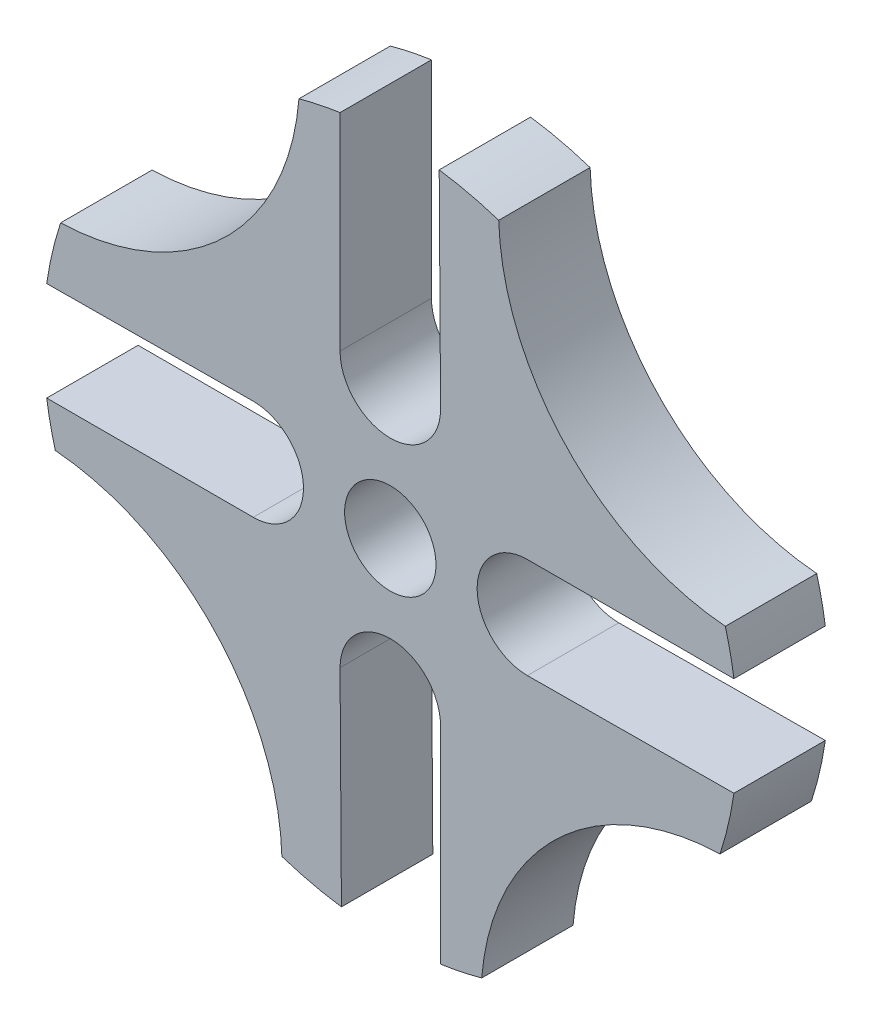
ISO-10303-21;
HEADER;
FILE_DESCRIPTION(('STEP AP214'),'2;1');
FILE_NAME('part.step','',(''),(''),'','','');
FILE_SCHEMA(('AUTOMOTIVE_DESIGN { 1 0 10303 214 1 1 1 1 }'));
ENDSEC;
DATA;
#1=APPLICATION_CONTEXT('core data for automotive mechanical design processes');
#2=APPLICATION_PROTOCOL_DEFINITION('international standard','automotive_design',2000,#1);
#3=PRODUCT_CONTEXT('',#1,'mechanical');
#4=PRODUCT('Part','Part','',(#3));
#5=PRODUCT_RELATED_PRODUCT_CATEGORY('part','',(#4));
#6=PRODUCT_DEFINITION_FORMATION('','',#4);
#7=PRODUCT_DEFINITION_CONTEXT('part definition',#1,'design');
#8=PRODUCT_DEFINITION('design','',#6,#7);
#9=PRODUCT_DEFINITION_SHAPE('','',#8);
#10=(LENGTH_UNIT() NAMED_UNIT(*) SI_UNIT(.MILLI.,.METRE.));
#11=(NAMED_UNIT(*) PLANE_ANGLE_UNIT() SI_UNIT($,.RADIAN.));
#12=(NAMED_UNIT(*) SI_UNIT($,.STERADIAN.) SOLID_ANGLE_UNIT());
#13=UNCERTAINTY_MEASURE_WITH_UNIT(LENGTH_MEASURE(1.E-05),#10,'distance_accuracy_value','');
#14=(GEOMETRIC_REPRESENTATION_CONTEXT(3) GLOBAL_UNCERTAINTY_ASSIGNED_CONTEXT((#13)) GLOBAL_UNIT_ASSIGNED_CONTEXT((#10,
#11,#12)) REPRESENTATION_CONTEXT('',''));
#15=CARTESIAN_POINT('',(0.,0.,0.));
#16=DIRECTION('',(0.,0.,1.));
#17=DIRECTION('',(1.,0.,0.));
#18=AXIS2_PLACEMENT_3D('',#15,#16,#17);
#19=CARTESIAN_POINT('',(-36.9110934311923,38.8499091789837,10.));
#20=DIRECTION('',(0.,0.,-1.));
#21=DIRECTION('',(-1.,0.,0.));
#22=AXIS2_PLACEMENT_3D('',#19,#20,#21);
#23=CYLINDRICAL_SURFACE('',#22,27.);
#24=CARTESIAN_POINT('',(-36.9110934311923,38.8499091789837,0.));
#25=DIRECTION('',(0.,0.,1.));
#26=DIRECTION('',(1.,0.,0.));
#27=AXIS2_PLACEMENT_3D('',#24,#25,#26);
#28=CIRCLE('',#27,27.);
#29=CARTESIAN_POINT('',(-36.078505424815,11.8627493207912,0.));
#30=VERTEX_POINT('',#29);
#31=CARTESIAN_POINT('',(-10.,36.6606055596466,0.));
#32=VERTEX_POINT('',#31);
#33=EDGE_CURVE('E239',#30,#32,#28,.T.);
#34=ORIENTED_EDGE('',*,*,#33,.F.);
#35=DIRECTION('',(0.,0.,-1.));
#36=VECTOR('',#35,1.);
#37=CARTESIAN_POINT('',(-36.078505424815,11.8627493207912,10.));
#38=LINE('',#37,#36);
#39=CARTESIAN_POINT('',(-36.078505424815,11.8627493207912,10.));
#40=VERTEX_POINT('',#39);
#41=EDGE_CURVE('E11',#40,#30,#38,.T.);
#42=ORIENTED_EDGE('',*,*,#41,.F.);
#43=CARTESIAN_POINT('',(-36.9110934311923,38.8499091789837,10.));
#44=DIRECTION('',(0.,0.,1.));
#45=DIRECTION('',(1.,0.,0.));
#46=AXIS2_PLACEMENT_3D('',#43,#44,#45);
#47=CIRCLE('',#46,27.);
#48=CARTESIAN_POINT('',(-10.,36.6606055596466,10.));
#49=VERTEX_POINT('',#48);
#50=EDGE_CURVE('E308',#40,#49,#47,.T.);
#51=ORIENTED_EDGE('',*,*,#50,.T.);
#52=DIRECTION('',(0.,0.,-1.));
#53=VECTOR('',#52,1.);
#54=CARTESIAN_POINT('',(-10.,36.6606055596466,10.));
#55=LINE('',#54,#53);
#56=EDGE_CURVE('E141',#49,#32,#55,.T.);
#57=ORIENTED_EDGE('',*,*,#56,.T.);
#58=EDGE_LOOP('',(#34,#42,#51,#57));
#59=FACE_BOUND('',#58,.T.);
#60=ADVANCED_FACE('F44',(#59),#23,.F.);
#61=CARTESIAN_POINT('',(0.,0.,10.));
#62=DIRECTION('',(0.,0.,-1.));
#63=DIRECTION('',(-1.,0.,0.));
#64=AXIS2_PLACEMENT_3D('',#61,#62,#63);
#65=CYLINDRICAL_SURFACE('',#64,37.9787226633063);
#66=CARTESIAN_POINT('',(0.,0.,0.));
#67=DIRECTION('',(0.,0.,1.));
#68=DIRECTION('',(1.,0.,0.));
#69=AXIS2_PLACEMENT_3D('',#66,#67,#68);
#70=CIRCLE('',#69,37.9787226633063);
#71=CARTESIAN_POINT('',(-37.6,5.35008178781775,0.));
#72=VERTEX_POINT('',#71);
#73=EDGE_CURVE('E245',#30,#72,#70,.T.);
#74=ORIENTED_EDGE('',*,*,#73,.T.);
#75=DIRECTION('',(0.,0.,-1.));
#76=VECTOR('',#75,1.);
#77=CARTESIAN_POINT('',(-37.6,5.35008178781775,10.));
#78=LINE('',#77,#76);
#79=CARTESIAN_POINT('',(-37.6,5.35008178781775,10.));
#80=VERTEX_POINT('',#79);
#81=EDGE_CURVE('E52',#80,#72,#78,.T.);
#82=ORIENTED_EDGE('',*,*,#81,.F.);
#83=CARTESIAN_POINT('',(0.,0.,10.));
#84=DIRECTION('',(0.,0.,1.));
#85=DIRECTION('',(1.,0.,0.));
#86=AXIS2_PLACEMENT_3D('',#83,#84,#85);
#87=CIRCLE('',#86,37.9787226633063);
#88=EDGE_CURVE('E367',#40,#80,#87,.T.);
#89=ORIENTED_EDGE('',*,*,#88,.F.);
#90=ORIENTED_EDGE('',*,*,#41,.T.);
#91=EDGE_LOOP('',(#74,#82,#89,#90));
#92=FACE_BOUND('',#91,.T.);
#93=ADVANCED_FACE('F360',(#92),#65,.T.);
#94=CARTESIAN_POINT('',(-0.0371429458533851,5.59925684861287,10.));
#95=DIRECTION('',(0.00663340326509993,-0.999977998738534,0.));
#96=DIRECTION('',(0.999977998738534,0.00663340326509993,0.));
#97=AXIS2_PLACEMENT_3D('',#94,#95,#96);
#98=PLANE('',#97);
#99=DIRECTION('',(-0.999977998738534,-0.00663340326509993,0.));
#100=VECTOR('',#99,1.);
#101=CARTESIAN_POINT('',(-0.0371429458533851,5.59925684861287,0.));
#102=LINE('',#101,#100);
#103=CARTESIAN_POINT('',(-14.9999999999998,5.4999999999988,0.));
#104=VERTEX_POINT('',#103);
#105=EDGE_CURVE('E243',#104,#72,#102,.T.);
#106=ORIENTED_EDGE('',*,*,#105,.F.);
#107=DIRECTION('',(0.,0.,-1.));
#108=VECTOR('',#107,1.);
#109=CARTESIAN_POINT('',(-14.9999999999998,5.4999999999988,10.));
#110=LINE('',#109,#108);
#111=CARTESIAN_POINT('',(-14.9999999999998,5.4999999999988,10.));
#112=VERTEX_POINT('',#111);
#113=EDGE_CURVE('E350',#112,#104,#110,.T.);
#114=ORIENTED_EDGE('',*,*,#113,.F.);
#115=DIRECTION('',(-0.999977998738534,-0.00663340326509993,0.));
#116=VECTOR('',#115,1.);
#117=CARTESIAN_POINT('',(-0.0371429458533851,5.59925684861287,10.));
#118=LINE('',#117,#116);
#119=EDGE_CURVE('E351',#112,#80,#118,.T.);
#120=ORIENTED_EDGE('',*,*,#119,.T.);
#121=ORIENTED_EDGE('',*,*,#81,.T.);
#122=EDGE_LOOP('',(#106,#114,#120,#121));
#123=FACE_BOUND('',#122,.T.);
#124=ADVANCED_FACE('F355',(#123),#98,.T.);
#125=CARTESIAN_POINT('',(-14.9999999999998,-1.20234347830044E-12,10.));
#126=DIRECTION('',(0.,0.,-1.));
#127=DIRECTION('',(-1.,0.,0.));
#128=AXIS2_PLACEMENT_3D('',#125,#126,#127);
#129=CYLINDRICAL_SURFACE('',#128,5.49999999999999);
#130=CARTESIAN_POINT('',(-14.9999999999998,-1.20234347830044E-12,0.));
#131=DIRECTION('',(0.,0.,1.));
#132=DIRECTION('',(1.,0.,0.));
#133=AXIS2_PLACEMENT_3D('',#130,#131,#132);
#134=CIRCLE('',#133,5.49999999999999);
#135=CARTESIAN_POINT('',(-14.9999999999998,-5.50000000000118,0.));
#136=VERTEX_POINT('',#135);
#137=EDGE_CURVE('E246',#136,#104,#134,.T.);
#138=ORIENTED_EDGE('',*,*,#137,.F.);
#139=DIRECTION('',(0.,0.,-1.));
#140=VECTOR('',#139,1.);
#141=CARTESIAN_POINT('',(-14.9999999999998,-5.50000000000118,10.));
#142=LINE('',#141,#140);
#143=CARTESIAN_POINT('',(-14.9999999999998,-5.50000000000118,10.));
#144=VERTEX_POINT('',#143);
#145=EDGE_CURVE('E342',#144,#136,#142,.T.);
#146=ORIENTED_EDGE('',*,*,#145,.F.);
#147=CARTESIAN_POINT('',(-14.9999999999998,-1.20234347830044E-12,10.));
#148=DIRECTION('',(0.,0.,1.));
#149=DIRECTION('',(1.,0.,0.));
#150=AXIS2_PLACEMENT_3D('',#147,#148,#149);
#151=CIRCLE('',#150,5.49999999999999);
#152=EDGE_CURVE('E369',#144,#112,#151,.T.);
#153=ORIENTED_EDGE('',*,*,#152,.T.);
#154=ORIENTED_EDGE('',*,*,#113,.T.);
#155=EDGE_LOOP('',(#138,#146,#153,#154));
#156=FACE_BOUND('',#155,.T.);
#157=ADVANCED_FACE('F364',(#156),#129,.F.);
#158=CARTESIAN_POINT('',(0.,-5.50000000000119,10.));
#159=DIRECTION('',(0.,-1.,0.));
#160=DIRECTION('',(1.,0.,0.));
#161=AXIS2_PLACEMENT_3D('',#158,#159,#160);
#162=PLANE('',#161);
#163=DIRECTION('',(-1.,0.,0.));
#164=VECTOR('',#163,1.);
#165=CARTESIAN_POINT('',(0.,-5.50000000000119,0.));
#166=LINE('',#165,#164);
#167=CARTESIAN_POINT('',(-37.5998670210413,-5.50000000000118,0.));
#168=VERTEX_POINT('',#167);
#169=EDGE_CURVE('E253',#136,#168,#166,.T.);
#170=ORIENTED_EDGE('',*,*,#169,.T.);
#171=DIRECTION('',(0.,0.,-1.));
#172=VECTOR('',#171,1.);
#173=CARTESIAN_POINT('',(-37.5998670210413,-5.50000000000118,10.));
#174=LINE('',#173,#172);
#175=CARTESIAN_POINT('',(-37.5998670210413,-5.50000000000118,10.));
#176=VERTEX_POINT('',#175);
#177=EDGE_CURVE('E345',#176,#168,#174,.T.);
#178=ORIENTED_EDGE('',*,*,#177,.F.);
#179=DIRECTION('',(-1.,0.,0.));
#180=VECTOR('',#179,1.);
#181=CARTESIAN_POINT('',(0.,-5.50000000000119,10.));
#182=LINE('',#181,#180);
#183=EDGE_CURVE('E375',#144,#176,#182,.T.);
#184=ORIENTED_EDGE('',*,*,#183,.F.);
#185=ORIENTED_EDGE('',*,*,#145,.T.);
#186=EDGE_LOOP('',(#170,#178,#184,#185));
#187=FACE_BOUND('',#186,.T.);
#188=ADVANCED_FACE('F434',(#187),#162,.F.);
#189=CARTESIAN_POINT('',(0.,0.,10.));
#190=DIRECTION('',(0.,0.,-1.));
#191=DIRECTION('',(-1.,0.,0.));
#192=AXIS2_PLACEMENT_3D('',#189,#190,#191);
#193=CYLINDRICAL_SURFACE('',#192,38.);
#194=CARTESIAN_POINT('',(0.,0.,0.));
#195=DIRECTION('',(0.,0.,1.));
#196=DIRECTION('',(1.,0.,0.));
#197=AXIS2_PLACEMENT_3D('',#194,#195,#196);
#198=CIRCLE('',#197,38.);
#199=CARTESIAN_POINT('',(-36.6606055596467,-10.,0.));
#200=VERTEX_POINT('',#199);
#201=EDGE_CURVE('E251',#168,#200,#198,.T.);
#202=ORIENTED_EDGE('',*,*,#201,.T.);
#203=DIRECTION('',(0.,0.,-1.));
#204=VECTOR('',#203,1.);
#205=CARTESIAN_POINT('',(-36.6606055596467,-10.,10.));
#206=LINE('',#205,#204);
#207=CARTESIAN_POINT('',(-36.6606055596467,-10.,10.));
#208=VERTEX_POINT('',#207);
#209=EDGE_CURVE('E338',#208,#200,#206,.T.);
#210=ORIENTED_EDGE('',*,*,#209,.F.);
#211=CARTESIAN_POINT('',(0.,0.,10.));
#212=DIRECTION('',(0.,0.,1.));
#213=DIRECTION('',(1.,0.,0.));
#214=AXIS2_PLACEMENT_3D('',#211,#212,#213);
#215=CIRCLE('',#214,38.);
#216=EDGE_CURVE('E378',#176,#208,#215,.T.);
#217=ORIENTED_EDGE('',*,*,#216,.F.);
#218=ORIENTED_EDGE('',*,*,#177,.T.);
#219=EDGE_LOOP('',(#202,#210,#217,#218));
#220=FACE_BOUND('',#219,.T.);
#221=ADVANCED_FACE('F437',(#220),#193,.T.);
#222=CARTESIAN_POINT('',(-38.8499091789837,-36.9110934311923,10.));
#223=DIRECTION('',(0.,0.,-1.));
#224=DIRECTION('',(-1.,0.,0.));
#225=AXIS2_PLACEMENT_3D('',#222,#223,#224);
#226=CYLINDRICAL_SURFACE('',#225,27.);
#227=CARTESIAN_POINT('',(-38.8499091789837,-36.9110934311923,0.));
#228=DIRECTION('',(0.,0.,1.));
#229=DIRECTION('',(1.,0.,0.));
#230=AXIS2_PLACEMENT_3D('',#227,#228,#229);
#231=CIRCLE('',#230,27.);
#232=CARTESIAN_POINT('',(-11.8627493207912,-36.078505424815,0.));
#233=VERTEX_POINT('',#232);
#234=EDGE_CURVE('E258',#233,#200,#231,.T.);
#235=ORIENTED_EDGE('',*,*,#234,.F.);
#236=DIRECTION('',(0.,0.,-1.));
#237=VECTOR('',#236,1.);
#238=CARTESIAN_POINT('',(-11.8627493207912,-36.078505424815,10.));
#239=LINE('',#238,#237);
#240=CARTESIAN_POINT('',(-11.8627493207912,-36.078505424815,10.));
#241=VERTEX_POINT('',#240);
#242=EDGE_CURVE('E339',#241,#233,#239,.T.);
#243=ORIENTED_EDGE('',*,*,#242,.F.);
#244=CARTESIAN_POINT('',(-38.8499091789837,-36.9110934311923,10.));
#245=DIRECTION('',(0.,0.,1.));
#246=DIRECTION('',(1.,0.,0.));
#247=AXIS2_PLACEMENT_3D('',#244,#245,#246);
#248=CIRCLE('',#247,27.);
#249=EDGE_CURVE('E379',#241,#208,#248,.T.);
#250=ORIENTED_EDGE('',*,*,#249,.T.);
#251=ORIENTED_EDGE('',*,*,#209,.T.);
#252=EDGE_LOOP('',(#235,#243,#250,#251));
#253=FACE_BOUND('',#252,.T.);
#254=ADVANCED_FACE('F445',(#253),#226,.F.);
#255=CARTESIAN_POINT('',(0.,0.,10.));
#256=DIRECTION('',(0.,0.,-1.));
#257=DIRECTION('',(-1.,0.,0.));
#258=AXIS2_PLACEMENT_3D('',#255,#256,#257);
#259=CYLINDRICAL_SURFACE('',#258,37.9787226633063);
#260=CARTESIAN_POINT('',(0.,0.,0.));
#261=DIRECTION('',(0.,0.,1.));
#262=DIRECTION('',(1.,0.,0.));
#263=AXIS2_PLACEMENT_3D('',#260,#261,#262);
#264=CIRCLE('',#263,37.9787226633063);
#265=CARTESIAN_POINT('',(-5.35008178781776,-37.6,0.));
#266=VERTEX_POINT('',#265);
#267=EDGE_CURVE('E259',#233,#266,#264,.T.);
#268=ORIENTED_EDGE('',*,*,#267,.T.);
#269=DIRECTION('',(0.,0.,-1.));
#270=VECTOR('',#269,1.);
#271=CARTESIAN_POINT('',(-5.35008178781776,-37.6,10.));
#272=LINE('',#271,#270);
#273=CARTESIAN_POINT('',(-5.35008178781776,-37.6,10.));
#274=VERTEX_POINT('',#273);
#275=EDGE_CURVE('E337',#274,#266,#272,.T.);
#276=ORIENTED_EDGE('',*,*,#275,.F.);
#277=CARTESIAN_POINT('',(0.,0.,10.));
#278=DIRECTION('',(0.,0.,1.));
#279=DIRECTION('',(1.,0.,0.));
#280=AXIS2_PLACEMENT_3D('',#277,#278,#279);
#281=CIRCLE('',#280,37.9787226633063);
#282=EDGE_CURVE('E382',#241,#274,#281,.T.);
#283=ORIENTED_EDGE('',*,*,#282,.F.);
#284=ORIENTED_EDGE('',*,*,#242,.T.);
#285=EDGE_LOOP('',(#268,#276,#283,#284));
#286=FACE_BOUND('',#285,.T.);
#287=ADVANCED_FACE('F447',(#286),#259,.T.);
#288=CARTESIAN_POINT('',(-5.59925684861487,-0.0371429458536963,10.));
#289=DIRECTION('',(0.999977998738533,0.00663340326515312,0.));
#290=DIRECTION('',(-0.00663340326515312,0.999977998738533,0.));
#291=AXIS2_PLACEMENT_3D('',#288,#289,#290);
#292=PLANE('',#291);
#293=DIRECTION('',(0.00663340326515312,-0.999977998738533,0.));
#294=VECTOR('',#293,1.);
#295=CARTESIAN_POINT('',(-5.59925684861487,-0.0371429458536963,0.));
#296=LINE('',#295,#294);
#297=CARTESIAN_POINT('',(-5.5,-15.,0.));
#298=VERTEX_POINT('',#297);
#299=EDGE_CURVE('E265',#298,#266,#296,.T.);
#300=ORIENTED_EDGE('',*,*,#299,.F.);
#301=DIRECTION('',(0.,0.,-1.));
#302=VECTOR('',#301,1.);
#303=CARTESIAN_POINT('',(-5.5,-15.,10.));
#304=LINE('',#303,#302);
#305=CARTESIAN_POINT('',(-5.5,-15.,10.));
#306=VERTEX_POINT('',#305);
#307=EDGE_CURVE('E331',#306,#298,#304,.T.);
#308=ORIENTED_EDGE('',*,*,#307,.F.);
#309=DIRECTION('',(0.00663340326515312,-0.999977998738533,0.));
#310=VECTOR('',#309,1.);
#311=CARTESIAN_POINT('',(-5.59925684861487,-0.0371429458536963,10.));
#312=LINE('',#311,#310);
#313=EDGE_CURVE('E384',#306,#274,#312,.T.);
#314=ORIENTED_EDGE('',*,*,#313,.T.);
#315=ORIENTED_EDGE('',*,*,#275,.T.);
#316=EDGE_LOOP('',(#300,#308,#314,#315));
#317=FACE_BOUND('',#316,.T.);
#318=ADVANCED_FACE('F448',(#317),#292,.T.);
#319=CARTESIAN_POINT('',(0.,-15.,10.));
#320=DIRECTION('',(0.,0.,-1.));
#321=DIRECTION('',(-1.,0.,0.));
#322=AXIS2_PLACEMENT_3D('',#319,#320,#321);
#323=CYLINDRICAL_SURFACE('',#322,5.5);
#324=CARTESIAN_POINT('',(0.,-15.,0.));
#325=DIRECTION('',(0.,0.,1.));
#326=DIRECTION('',(1.,0.,0.));
#327=AXIS2_PLACEMENT_3D('',#324,#325,#326);
#328=CIRCLE('',#327,5.5);
#329=CARTESIAN_POINT('',(5.5,-15.,0.));
#330=VERTEX_POINT('',#329);
#331=EDGE_CURVE('E264',#330,#298,#328,.T.);
#332=ORIENTED_EDGE('',*,*,#331,.F.);
#333=DIRECTION('',(0.,0.,-1.));
#334=VECTOR('',#333,1.);
#335=CARTESIAN_POINT('',(5.5,-15.,10.));
#336=LINE('',#335,#334);
#337=CARTESIAN_POINT('',(5.5,-15.,10.));
#338=VERTEX_POINT('',#337);
#339=EDGE_CURVE('E335',#338,#330,#336,.T.);
#340=ORIENTED_EDGE('',*,*,#339,.F.);
#341=CARTESIAN_POINT('',(0.,-15.,10.));
#342=DIRECTION('',(0.,0.,1.));
#343=DIRECTION('',(1.,0.,0.));
#344=AXIS2_PLACEMENT_3D('',#341,#342,#343);
#345=CIRCLE('',#344,5.5);
#346=EDGE_CURVE('E389',#338,#306,#345,.T.);
#347=ORIENTED_EDGE('',*,*,#346,.T.);
#348=ORIENTED_EDGE('',*,*,#307,.T.);
#349=EDGE_LOOP('',(#332,#340,#347,#348));
#350=FACE_BOUND('',#349,.T.);
#351=ADVANCED_FACE('F454',(#350),#323,.F.);
#352=CARTESIAN_POINT('',(5.5,0.,10.));
#353=DIRECTION('',(1.,0.,0.));
#354=DIRECTION('',(0.,1.,0.));
#355=AXIS2_PLACEMENT_3D('',#352,#353,#354);
#356=PLANE('',#355);
#357=DIRECTION('',(0.,-1.,0.));
#358=VECTOR('',#357,1.);
#359=CARTESIAN_POINT('',(5.5,0.,0.));
#360=LINE('',#359,#358);
#361=CARTESIAN_POINT('',(5.5,-37.5998670210414,0.));
#362=VERTEX_POINT('',#361);
#363=EDGE_CURVE('E268',#330,#362,#360,.T.);
#364=ORIENTED_EDGE('',*,*,#363,.T.);
#365=DIRECTION('',(0.,0.,-1.));
#366=VECTOR('',#365,1.);
#367=CARTESIAN_POINT('',(5.5,-37.5998670210414,10.));
#368=LINE('',#367,#366);
#369=CARTESIAN_POINT('',(5.5,-37.5998670210414,10.));
#370=VERTEX_POINT('',#369);
#371=EDGE_CURVE('E328',#370,#362,#368,.T.);
#372=ORIENTED_EDGE('',*,*,#371,.F.);
#373=DIRECTION('',(0.,-1.,0.));
#374=VECTOR('',#373,1.);
#375=CARTESIAN_POINT('',(5.5,0.,10.));
#376=LINE('',#375,#374);
#377=EDGE_CURVE('E392',#338,#370,#376,.T.);
#378=ORIENTED_EDGE('',*,*,#377,.F.);
#379=ORIENTED_EDGE('',*,*,#339,.T.);
#380=EDGE_LOOP('',(#364,#372,#378,#379));
#381=FACE_BOUND('',#380,.T.);
#382=ADVANCED_FACE('F456',(#381),#356,.F.);
#383=CARTESIAN_POINT('',(0.,0.,10.));
#384=DIRECTION('',(0.,0.,-1.));
#385=DIRECTION('',(-1.,0.,0.));
#386=AXIS2_PLACEMENT_3D('',#383,#384,#385);
#387=CYLINDRICAL_SURFACE('',#386,38.);
#388=CARTESIAN_POINT('',(0.,0.,0.));
#389=DIRECTION('',(0.,0.,1.));
#390=DIRECTION('',(1.,0.,0.));
#391=AXIS2_PLACEMENT_3D('',#388,#389,#390);
#392=CIRCLE('',#391,38.);
#393=CARTESIAN_POINT('',(10.,-36.6606055596467,0.));
#394=VERTEX_POINT('',#393);
#395=EDGE_CURVE('E269',#362,#394,#392,.T.);
#396=ORIENTED_EDGE('',*,*,#395,.T.);
#397=DIRECTION('',(0.,0.,-1.));
#398=VECTOR('',#397,1.);
#399=CARTESIAN_POINT('',(10.,-36.6606055596467,10.));
#400=LINE('',#399,#398);
#401=CARTESIAN_POINT('',(10.,-36.6606055596467,10.));
#402=VERTEX_POINT('',#401);
#403=EDGE_CURVE('E330',#402,#394,#400,.T.);
#404=ORIENTED_EDGE('',*,*,#403,.F.);
#405=CARTESIAN_POINT('',(0.,0.,10.));
#406=DIRECTION('',(0.,0.,1.));
#407=DIRECTION('',(1.,0.,0.));
#408=AXIS2_PLACEMENT_3D('',#405,#406,#407);
#409=CIRCLE('',#408,38.);
#410=EDGE_CURVE('E394',#370,#402,#409,.T.);
#411=ORIENTED_EDGE('',*,*,#410,.F.);
#412=ORIENTED_EDGE('',*,*,#371,.T.);
#413=EDGE_LOOP('',(#396,#404,#411,#412));
#414=FACE_BOUND('',#413,.T.);
#415=ADVANCED_FACE('F465',(#414),#387,.T.);
#416=CARTESIAN_POINT('',(36.9110934311923,-38.8499091789837,10.));
#417=DIRECTION('',(0.,0.,-1.));
#418=DIRECTION('',(-1.,0.,0.));
#419=AXIS2_PLACEMENT_3D('',#416,#417,#418);
#420=CYLINDRICAL_SURFACE('',#419,27.);
#421=CARTESIAN_POINT('',(36.9110934311923,-38.8499091789837,0.));
#422=DIRECTION('',(0.,0.,1.));
#423=DIRECTION('',(1.,0.,0.));
#424=AXIS2_PLACEMENT_3D('',#421,#422,#423);
#425=CIRCLE('',#424,27.);
#426=CARTESIAN_POINT('',(36.078505424815,-11.8627493207912,0.));
#427=VERTEX_POINT('',#426);
#428=EDGE_CURVE('E272',#427,#394,#425,.T.);
#429=ORIENTED_EDGE('',*,*,#428,.F.);
#430=DIRECTION('',(0.,0.,-1.));
#431=VECTOR('',#430,1.);
#432=CARTESIAN_POINT('',(36.078505424815,-11.8627493207912,10.));
#433=LINE('',#432,#431);
#434=CARTESIAN_POINT('',(36.078505424815,-11.8627493207912,10.));
#435=VERTEX_POINT('',#434);
#436=EDGE_CURVE('E324',#435,#427,#433,.T.);
#437=ORIENTED_EDGE('',*,*,#436,.F.);
#438=CARTESIAN_POINT('',(36.9110934311923,-38.8499091789837,10.));
#439=DIRECTION('',(0.,0.,1.));
#440=DIRECTION('',(1.,0.,0.));
#441=AXIS2_PLACEMENT_3D('',#438,#439,#440);
#442=CIRCLE('',#441,27.);
#443=EDGE_CURVE('E393',#435,#402,#442,.T.);
#444=ORIENTED_EDGE('',*,*,#443,.T.);
#445=ORIENTED_EDGE('',*,*,#403,.T.);
#446=EDGE_LOOP('',(#429,#437,#444,#445));
#447=FACE_BOUND('',#446,.T.);
#448=ADVANCED_FACE('F468',(#447),#420,.F.);
#449=CARTESIAN_POINT('',(0.,0.,10.));
#450=DIRECTION('',(0.,0.,-1.));
#451=DIRECTION('',(-1.,0.,0.));
#452=AXIS2_PLACEMENT_3D('',#449,#450,#451);
#453=CYLINDRICAL_SURFACE('',#452,37.9787226633063);
#454=CARTESIAN_POINT('',(0.,0.,0.));
#455=DIRECTION('',(0.,0.,1.));
#456=DIRECTION('',(1.,0.,0.));
#457=AXIS2_PLACEMENT_3D('',#454,#455,#456);
#458=CIRCLE('',#457,37.9787226633063);
#459=CARTESIAN_POINT('',(37.6,-5.35008178781776,0.));
#460=VERTEX_POINT('',#459);
#461=EDGE_CURVE('E277',#427,#460,#458,.T.);
#462=ORIENTED_EDGE('',*,*,#461,.T.);
#463=DIRECTION('',(0.,0.,-1.));
#464=VECTOR('',#463,1.);
#465=CARTESIAN_POINT('',(37.6,-5.35008178781776,10.));
#466=LINE('',#465,#464);
#467=CARTESIAN_POINT('',(37.6,-5.35008178781776,10.));
#468=VERTEX_POINT('',#467);
#469=EDGE_CURVE('E323',#468,#460,#466,.T.);
#470=ORIENTED_EDGE('',*,*,#469,.F.);
#471=CARTESIAN_POINT('',(0.,0.,10.));
#472=DIRECTION('',(0.,0.,1.));
#473=DIRECTION('',(1.,0.,0.));
#474=AXIS2_PLACEMENT_3D('',#471,#472,#473);
#475=CIRCLE('',#474,37.9787226633063);
#476=EDGE_CURVE('E396',#435,#468,#475,.T.);
#477=ORIENTED_EDGE('',*,*,#476,.F.);
#478=ORIENTED_EDGE('',*,*,#436,.T.);
#479=EDGE_LOOP('',(#462,#470,#477,#478));
#480=FACE_BOUND('',#479,.T.);
#481=ADVANCED_FACE('F467',(#480),#453,.T.);
#482=CARTESIAN_POINT('',(0.0371429458536561,-5.59925684861462,10.));
#483=DIRECTION('',(-0.00663340326514626,0.999977998738533,0.));
#484=DIRECTION('',(-0.999977998738533,-0.00663340326514626,0.));
#485=AXIS2_PLACEMENT_3D('',#482,#483,#484);
#486=PLANE('',#485);
#487=DIRECTION('',(0.999977998738533,0.00663340326514626,0.));
#488=VECTOR('',#487,1.);
#489=CARTESIAN_POINT('',(0.0371429458536561,-5.59925684861462,0.));
#490=LINE('',#489,#488);
#491=CARTESIAN_POINT('',(15.0000000000012,-5.49999999999984,0.));
#492=VERTEX_POINT('',#491);
#493=EDGE_CURVE('E276',#492,#460,#490,.T.);
#494=ORIENTED_EDGE('',*,*,#493,.F.);
#495=DIRECTION('',(0.,0.,-1.));
#496=VECTOR('',#495,1.);
#497=CARTESIAN_POINT('',(15.0000000000012,-5.49999999999984,10.));
#498=LINE('',#497,#496);
#499=CARTESIAN_POINT('',(15.0000000000012,-5.49999999999984,10.));
#500=VERTEX_POINT('',#499);
#501=EDGE_CURVE('E321',#500,#492,#498,.T.);
#502=ORIENTED_EDGE('',*,*,#501,.F.);
#503=DIRECTION('',(0.999977998738533,0.00663340326514626,0.));
#504=VECTOR('',#503,1.);
#505=CARTESIAN_POINT('',(0.0371429458536561,-5.59925684861462,10.));
#506=LINE('',#505,#504);
#507=EDGE_CURVE('E397',#500,#468,#506,.T.);
#508=ORIENTED_EDGE('',*,*,#507,.T.);
#509=ORIENTED_EDGE('',*,*,#469,.T.);
#510=EDGE_LOOP('',(#494,#502,#508,#509));
#511=FACE_BOUND('',#510,.T.);
#512=ADVANCED_FACE('F475',(#511),#486,.T.);
#513=CARTESIAN_POINT('',(15.0000000000012,1.59672422515636E-13,10.));
#514=DIRECTION('',(0.,0.,-1.));
#515=DIRECTION('',(-1.,0.,0.));
#516=AXIS2_PLACEMENT_3D('',#513,#514,#515);
#517=CYLINDRICAL_SURFACE('',#516,5.49999999999999);
#518=CARTESIAN_POINT('',(15.0000000000012,1.59672422515636E-13,0.));
#519=DIRECTION('',(0.,0.,1.));
#520=DIRECTION('',(1.,0.,0.));
#521=AXIS2_PLACEMENT_3D('',#518,#519,#520);
#522=CIRCLE('',#521,5.49999999999999);
#523=CARTESIAN_POINT('',(15.0000000000012,5.50000000000014,0.));
#524=VERTEX_POINT('',#523);
#525=EDGE_CURVE('E285',#524,#492,#522,.T.);
#526=ORIENTED_EDGE('',*,*,#525,.F.);
#527=DIRECTION('',(0.,0.,-1.));
#528=VECTOR('',#527,1.);
#529=CARTESIAN_POINT('',(15.0000000000012,5.50000000000014,10.));
#530=LINE('',#529,#528);
#531=CARTESIAN_POINT('',(15.0000000000012,5.50000000000014,10.));
#532=VERTEX_POINT('',#531);
#533=EDGE_CURVE('E317',#532,#524,#530,.T.);
#534=ORIENTED_EDGE('',*,*,#533,.F.);
#535=CARTESIAN_POINT('',(15.0000000000012,1.59672422515636E-13,10.));
#536=DIRECTION('',(0.,0.,1.));
#537=DIRECTION('',(1.,0.,0.));
#538=AXIS2_PLACEMENT_3D('',#535,#536,#537);
#539=CIRCLE('',#538,5.49999999999999);
#540=EDGE_CURVE('E401',#532,#500,#539,.T.);
#541=ORIENTED_EDGE('',*,*,#540,.T.);
#542=ORIENTED_EDGE('',*,*,#501,.T.);
#543=EDGE_LOOP('',(#526,#534,#541,#542));
#544=FACE_BOUND('',#543,.T.);
#545=ADVANCED_FACE('F476',(#544),#517,.F.);
#546=CARTESIAN_POINT('',(0.,5.50000000000013,10.));
#547=DIRECTION('',(0.,1.,0.));
#548=DIRECTION('',(-1.,0.,0.));
#549=AXIS2_PLACEMENT_3D('',#546,#547,#548);
#550=PLANE('',#549);
#551=DIRECTION('',(1.,0.,0.));
#552=VECTOR('',#551,1.);
#553=CARTESIAN_POINT('',(0.,5.50000000000013,0.));
#554=LINE('',#553,#552);
#555=CARTESIAN_POINT('',(37.5998670210426,5.50000000000016,0.));
#556=VERTEX_POINT('',#555);
#557=EDGE_CURVE('E283',#524,#556,#554,.T.);
#558=ORIENTED_EDGE('',*,*,#557,.T.);
#559=DIRECTION('',(0.,0.,-1.));
#560=VECTOR('',#559,1.);
#561=CARTESIAN_POINT('',(37.5998670210426,5.50000000000016,10.));
#562=LINE('',#561,#560);
#563=CARTESIAN_POINT('',(37.5998670210426,5.50000000000016,10.));
#564=VERTEX_POINT('',#563);
#565=EDGE_CURVE('E316',#564,#556,#562,.T.);
#566=ORIENTED_EDGE('',*,*,#565,.F.);
#567=DIRECTION('',(1.,0.,0.));
#568=VECTOR('',#567,1.);
#569=CARTESIAN_POINT('',(0.,5.50000000000013,10.));
#570=LINE('',#569,#568);
#571=EDGE_CURVE('E407',#532,#564,#570,.T.);
#572=ORIENTED_EDGE('',*,*,#571,.F.);
#573=ORIENTED_EDGE('',*,*,#533,.T.);
#574=EDGE_LOOP('',(#558,#566,#572,#573));
#575=FACE_BOUND('',#574,.T.);
#576=ADVANCED_FACE('F485',(#575),#550,.F.);
#577=CARTESIAN_POINT('',(0.,0.,10.));
#578=DIRECTION('',(0.,0.,-1.));
#579=DIRECTION('',(-1.,0.,0.));
#580=AXIS2_PLACEMENT_3D('',#577,#578,#579);
#581=CYLINDRICAL_SURFACE('',#580,38.0000000000006);
#582=CARTESIAN_POINT('',(0.,0.,0.));
#583=DIRECTION('',(0.,0.,1.));
#584=DIRECTION('',(1.,0.,0.));
#585=AXIS2_PLACEMENT_3D('',#582,#583,#584);
#586=CIRCLE('',#585,38.0000000000006);
#587=CARTESIAN_POINT('',(36.6606055596473,10.0000000000002,0.));
#588=VERTEX_POINT('',#587);
#589=EDGE_CURVE('E290',#556,#588,#586,.T.);
#590=ORIENTED_EDGE('',*,*,#589,.T.);
#591=DIRECTION('',(0.,0.,-1.));
#592=VECTOR('',#591,1.);
#593=CARTESIAN_POINT('',(36.6606055596473,10.0000000000002,10.));
#594=LINE('',#593,#592);
#595=CARTESIAN_POINT('',(36.6606055596473,10.0000000000002,10.));
#596=VERTEX_POINT('',#595);
#597=EDGE_CURVE('E314',#596,#588,#594,.T.);
#598=ORIENTED_EDGE('',*,*,#597,.F.);
#599=CARTESIAN_POINT('',(0.,0.,10.));
#600=DIRECTION('',(0.,0.,1.));
#601=DIRECTION('',(1.,0.,0.));
#602=AXIS2_PLACEMENT_3D('',#599,#600,#601);
#603=CIRCLE('',#602,38.0000000000006);
#604=EDGE_CURVE('E409',#564,#596,#603,.T.);
#605=ORIENTED_EDGE('',*,*,#604,.F.);
#606=ORIENTED_EDGE('',*,*,#565,.T.);
#607=EDGE_LOOP('',(#590,#598,#605,#606));
#608=FACE_BOUND('',#607,.T.);
#609=ADVANCED_FACE('F486',(#608),#581,.T.);
#610=CARTESIAN_POINT('',(38.8499091789837,36.9110934311923,10.));
#611=DIRECTION('',(0.,0.,-1.));
#612=DIRECTION('',(-1.,0.,0.));
#613=AXIS2_PLACEMENT_3D('',#610,#611,#612);
#614=CYLINDRICAL_SURFACE('',#613,27.);
#615=CARTESIAN_POINT('',(38.8499091789837,36.9110934311923,0.));
#616=DIRECTION('',(0.,0.,1.));
#617=DIRECTION('',(1.,0.,0.));
#618=AXIS2_PLACEMENT_3D('',#615,#616,#617);
#619=CIRCLE('',#618,27.);
#620=CARTESIAN_POINT('',(11.8627493207912,36.078505424815,0.));
#621=VERTEX_POINT('',#620);
#622=EDGE_CURVE('E287',#621,#588,#619,.T.);
#623=ORIENTED_EDGE('',*,*,#622,.F.);
#624=DIRECTION('',(0.,0.,-1.));
#625=VECTOR('',#624,1.);
#626=CARTESIAN_POINT('',(11.8627493207912,36.078505424815,10.));
#627=LINE('',#626,#625);
#628=CARTESIAN_POINT('',(11.8627493207912,36.078505424815,10.));
#629=VERTEX_POINT('',#628);
#630=EDGE_CURVE('E315',#629,#621,#627,.T.);
#631=ORIENTED_EDGE('',*,*,#630,.F.);
#632=CARTESIAN_POINT('',(38.8499091789837,36.9110934311923,10.));
#633=DIRECTION('',(0.,0.,1.));
#634=DIRECTION('',(1.,0.,0.));
#635=AXIS2_PLACEMENT_3D('',#632,#633,#634);
#636=CIRCLE('',#635,27.);
#637=EDGE_CURVE('E408',#629,#596,#636,.T.);
#638=ORIENTED_EDGE('',*,*,#637,.T.);
#639=ORIENTED_EDGE('',*,*,#597,.T.);
#640=EDGE_LOOP('',(#623,#631,#638,#639));
#641=FACE_BOUND('',#640,.T.);
#642=ADVANCED_FACE('F489',(#641),#614,.F.);
#643=CARTESIAN_POINT('',(0.,0.,10.));
#644=DIRECTION('',(0.,0.,-1.));
#645=DIRECTION('',(-1.,0.,0.));
#646=AXIS2_PLACEMENT_3D('',#643,#644,#645);
#647=CYLINDRICAL_SURFACE('',#646,37.9787226633063);
#648=CARTESIAN_POINT('',(0.,0.,0.));
#649=DIRECTION('',(0.,0.,1.));
#650=DIRECTION('',(1.,0.,0.));
#651=AXIS2_PLACEMENT_3D('',#648,#649,#650);
#652=CIRCLE('',#651,37.9787226633063);
#653=CARTESIAN_POINT('',(5.35008178781776,37.6,0.));
#654=VERTEX_POINT('',#653);
#655=EDGE_CURVE('E291',#621,#654,#652,.T.);
#656=ORIENTED_EDGE('',*,*,#655,.T.);
#657=DIRECTION('',(0.,0.,-1.));
#658=VECTOR('',#657,1.);
#659=CARTESIAN_POINT('',(5.35008178781776,37.6,10.));
#660=LINE('',#659,#658);
#661=CARTESIAN_POINT('',(5.35008178781776,37.6,10.));
#662=VERTEX_POINT('',#661);
#663=EDGE_CURVE('E309',#662,#654,#660,.T.);
#664=ORIENTED_EDGE('',*,*,#663,.F.);
#665=CARTESIAN_POINT('',(0.,0.,10.));
#666=DIRECTION('',(0.,0.,1.));
#667=DIRECTION('',(1.,0.,0.));
#668=AXIS2_PLACEMENT_3D('',#665,#666,#667);
#669=CIRCLE('',#668,37.9787226633063);
#670=EDGE_CURVE('E233',#629,#662,#669,.T.);
#671=ORIENTED_EDGE('',*,*,#670,.F.);
#672=ORIENTED_EDGE('',*,*,#630,.T.);
#673=EDGE_LOOP('',(#656,#664,#671,#672));
#674=FACE_BOUND('',#673,.T.);
#675=ADVANCED_FACE('F418',(#674),#647,.T.);
#676=CARTESIAN_POINT('',(5.59925684861486,0.0371429458536938,10.));
#677=DIRECTION('',(-0.999977998738533,-0.0066334032651527,0.));
#678=DIRECTION('',(0.0066334032651527,-0.999977998738533,0.));
#679=AXIS2_PLACEMENT_3D('',#676,#677,#678);
#680=PLANE('',#679);
#681=DIRECTION('',(-0.0066334032651527,0.999977998738533,0.));
#682=VECTOR('',#681,1.);
#683=CARTESIAN_POINT('',(5.59925684861486,0.0371429458536938,0.));
#684=LINE('',#683,#682);
#685=CARTESIAN_POINT('',(5.5,15.,0.));
#686=VERTEX_POINT('',#685);
#687=EDGE_CURVE('E297',#686,#654,#684,.T.);
#688=ORIENTED_EDGE('',*,*,#687,.F.);
#689=DIRECTION('',(0.,0.,-1.));
#690=VECTOR('',#689,1.);
#691=CARTESIAN_POINT('',(5.5,15.,10.));
#692=LINE('',#691,#690);
#693=CARTESIAN_POINT('',(5.5,15.,10.));
#694=VERTEX_POINT('',#693);
#695=EDGE_CURVE('E218',#694,#686,#692,.T.);
#696=ORIENTED_EDGE('',*,*,#695,.F.);
#697=DIRECTION('',(-0.0066334032651527,0.999977998738533,0.));
#698=VECTOR('',#697,1.);
#699=CARTESIAN_POINT('',(5.59925684861486,0.0371429458536938,10.));
#700=LINE('',#699,#698);
#701=EDGE_CURVE('E226',#694,#662,#700,.T.);
#702=ORIENTED_EDGE('',*,*,#701,.T.);
#703=ORIENTED_EDGE('',*,*,#663,.T.);
#704=EDGE_LOOP('',(#688,#696,#702,#703));
#705=FACE_BOUND('',#704,.T.);
#706=ADVANCED_FACE('F419',(#705),#680,.T.);
#707=CARTESIAN_POINT('',(0.,15.,10.));
#708=DIRECTION('',(0.,0.,-1.));
#709=DIRECTION('',(-1.,0.,0.));
#710=AXIS2_PLACEMENT_3D('',#707,#708,#709);
#711=CYLINDRICAL_SURFACE('',#710,5.5);
#712=CARTESIAN_POINT('',(0.,15.,0.));
#713=DIRECTION('',(0.,0.,1.));
#714=DIRECTION('',(1.,0.,0.));
#715=AXIS2_PLACEMENT_3D('',#712,#713,#714);
#716=CIRCLE('',#715,5.5);
#717=CARTESIAN_POINT('',(-5.5,15.,0.));
#718=VERTEX_POINT('',#717);
#719=EDGE_CURVE('E217',#718,#686,#716,.T.);
#720=ORIENTED_EDGE('',*,*,#719,.F.);
#721=DIRECTION('',(0.,0.,-1.));
#722=VECTOR('',#721,1.);
#723=CARTESIAN_POINT('',(-5.5,15.,10.));
#724=LINE('',#723,#722);
#725=CARTESIAN_POINT('',(-5.5,15.,10.));
#726=VERTEX_POINT('',#725);
#727=EDGE_CURVE('E215',#726,#718,#724,.T.);
#728=ORIENTED_EDGE('',*,*,#727,.F.);
#729=CARTESIAN_POINT('',(0.,15.,10.));
#730=DIRECTION('',(0.,0.,1.));
#731=DIRECTION('',(1.,0.,0.));
#732=AXIS2_PLACEMENT_3D('',#729,#730,#731);
#733=CIRCLE('',#732,5.5);
#734=EDGE_CURVE('E216',#726,#694,#733,.T.);
#735=ORIENTED_EDGE('',*,*,#734,.T.);
#736=ORIENTED_EDGE('',*,*,#695,.T.);
#737=EDGE_LOOP('',(#720,#728,#735,#736));
#738=FACE_BOUND('',#737,.T.);
#739=ADVANCED_FACE('F212',(#738),#711,.F.);
#740=CARTESIAN_POINT('',(-5.5,0.,10.));
#741=DIRECTION('',(-1.,0.,0.));
#742=DIRECTION('',(0.,0.,1.));
#743=AXIS2_PLACEMENT_3D('',#740,#741,#742);
#744=PLANE('',#743);
#745=DIRECTION('',(0.,1.,0.));
#746=VECTOR('',#745,1.);
#747=CARTESIAN_POINT('',(-5.5,0.,0.));
#748=LINE('',#747,#746);
#749=CARTESIAN_POINT('',(-5.5,37.5998670210414,0.));
#750=VERTEX_POINT('',#749);
#751=EDGE_CURVE('E138',#718,#750,#748,.T.);
#752=ORIENTED_EDGE('',*,*,#751,.T.);
#753=DIRECTION('',(0.,0.,-1.));
#754=VECTOR('',#753,1.);
#755=CARTESIAN_POINT('',(-5.5,37.5998670210414,10.));
#756=LINE('',#755,#754);
#757=CARTESIAN_POINT('',(-5.5,37.5998670210414,10.));
#758=VERTEX_POINT('',#757);
#759=EDGE_CURVE('E219',#758,#750,#756,.T.);
#760=ORIENTED_EDGE('',*,*,#759,.F.);
#761=DIRECTION('',(0.,1.,0.));
#762=VECTOR('',#761,1.);
#763=CARTESIAN_POINT('',(-5.5,0.,10.));
#764=LINE('',#763,#762);
#765=EDGE_CURVE('E225',#726,#758,#764,.T.);
#766=ORIENTED_EDGE('',*,*,#765,.F.);
#767=ORIENTED_EDGE('',*,*,#727,.T.);
#768=EDGE_LOOP('',(#752,#760,#766,#767));
#769=FACE_BOUND('',#768,.T.);
#770=ADVANCED_FACE('F224',(#769),#744,.F.);
#771=CARTESIAN_POINT('',(0.,0.,10.));
#772=DIRECTION('',(0.,0.,-1.));
#773=DIRECTION('',(-1.,0.,0.));
#774=AXIS2_PLACEMENT_3D('',#771,#772,#773);
#775=CYLINDRICAL_SURFACE('',#774,37.9999999999999);
#776=CARTESIAN_POINT('',(0.,0.,0.));
#777=DIRECTION('',(0.,0.,1.));
#778=DIRECTION('',(1.,0.,0.));
#779=AXIS2_PLACEMENT_3D('',#776,#777,#778);
#780=CIRCLE('',#779,37.9999999999999);
#781=EDGE_CURVE('E303',#750,#32,#780,.T.);
#782=ORIENTED_EDGE('',*,*,#781,.T.);
#783=ORIENTED_EDGE('',*,*,#56,.F.);
#784=CARTESIAN_POINT('',(0.,0.,10.));
#785=DIRECTION('',(0.,0.,1.));
#786=DIRECTION('',(1.,0.,0.));
#787=AXIS2_PLACEMENT_3D('',#784,#785,#786);
#788=CIRCLE('',#787,37.9999999999999);
#789=EDGE_CURVE('E62',#758,#49,#788,.T.);
#790=ORIENTED_EDGE('',*,*,#789,.F.);
#791=ORIENTED_EDGE('',*,*,#759,.T.);
#792=EDGE_LOOP('',(#782,#783,#790,#791));
#793=FACE_BOUND('',#792,.T.);
#794=ADVANCED_FACE('F421',(#793),#775,.T.);
#795=CARTESIAN_POINT('',(0.,0.,10.));
#796=DIRECTION('',(0.,0.,-1.));
#797=DIRECTION('',(-1.,0.,0.));
#798=AXIS2_PLACEMENT_3D('',#795,#796,#797);
#799=CYLINDRICAL_SURFACE('',#798,5.);
#800=CARTESIAN_POINT('',(0.,0.,10.));
#801=DIRECTION('',(0.,0.,1.));
#802=DIRECTION('',(1.,0.,0.));
#803=AXIS2_PLACEMENT_3D('',#800,#801,#802);
#804=CIRCLE('',#803,5.);
#805=CARTESIAN_POINT('',(5.,0.,10.));
#806=VERTEX_POINT('',#805);
#807=EDGE_CURVE('E237',#806,#806,#804,.T.);
#808=ORIENTED_EDGE('',*,*,#807,.T.);
#809=EDGE_LOOP('',(#808));
#810=FACE_BOUND('',#809,.T.);
#811=CARTESIAN_POINT('',(0.,0.,0.));
#812=DIRECTION('',(0.,0.,1.));
#813=DIRECTION('',(1.,0.,0.));
#814=AXIS2_PLACEMENT_3D('',#811,#812,#813);
#815=CIRCLE('',#814,5.);
#816=CARTESIAN_POINT('',(5.,0.,0.));
#817=VERTEX_POINT('',#816);
#818=EDGE_CURVE('E301',#817,#817,#815,.T.);
#819=ORIENTED_EDGE('',*,*,#818,.F.);
#820=EDGE_LOOP('',(#819));
#821=FACE_BOUND('',#820,.T.);
#822=ADVANCED_FACE('F503',(#810,#821),#799,.F.);
#823=CARTESIAN_POINT('',(0.,0.,10.));
#824=DIRECTION('',(0.,0.,1.));
#825=DIRECTION('',(1.,0.,0.));
#826=AXIS2_PLACEMENT_3D('',#823,#824,#825);
#827=PLANE('',#826);
#828=ORIENTED_EDGE('',*,*,#50,.F.);
#829=ORIENTED_EDGE('',*,*,#88,.T.);
#830=ORIENTED_EDGE('',*,*,#119,.F.);
#831=ORIENTED_EDGE('',*,*,#152,.F.);
#832=ORIENTED_EDGE('',*,*,#183,.T.);
#833=ORIENTED_EDGE('',*,*,#216,.T.);
#834=ORIENTED_EDGE('',*,*,#249,.F.);
#835=ORIENTED_EDGE('',*,*,#282,.T.);
#836=ORIENTED_EDGE('',*,*,#313,.F.);
#837=ORIENTED_EDGE('',*,*,#346,.F.);
#838=ORIENTED_EDGE('',*,*,#377,.T.);
#839=ORIENTED_EDGE('',*,*,#410,.T.);
#840=ORIENTED_EDGE('',*,*,#443,.F.);
#841=ORIENTED_EDGE('',*,*,#476,.T.);
#842=ORIENTED_EDGE('',*,*,#507,.F.);
#843=ORIENTED_EDGE('',*,*,#540,.F.);
#844=ORIENTED_EDGE('',*,*,#571,.T.);
#845=ORIENTED_EDGE('',*,*,#604,.T.);
#846=ORIENTED_EDGE('',*,*,#637,.F.);
#847=ORIENTED_EDGE('',*,*,#670,.T.);
#848=ORIENTED_EDGE('',*,*,#701,.F.);
#849=ORIENTED_EDGE('',*,*,#734,.F.);
#850=ORIENTED_EDGE('',*,*,#765,.T.);
#851=ORIENTED_EDGE('',*,*,#789,.T.);
#852=EDGE_LOOP('',(#828,#829,#830,#831,#832,#833,#834,#835,#836,#837,#838,#839,#840,#841,#842,
#843,#844,#845,#846,#847,#848,#849,#850,#851));
#853=FACE_BOUND('',#852,.T.);
#854=ORIENTED_EDGE('',*,*,#807,.F.);
#855=EDGE_LOOP('',(#854));
#856=FACE_BOUND('',#855,.T.);
#857=ADVANCED_FACE('F227',(#853,#856),#827,.T.);
#858=CARTESIAN_POINT('',(0.,0.,0.));
#859=DIRECTION('',(0.,0.,1.));
#860=DIRECTION('',(1.,0.,0.));
#861=AXIS2_PLACEMENT_3D('',#858,#859,#860);
#862=PLANE('',#861);
#863=ORIENTED_EDGE('',*,*,#33,.T.);
#864=ORIENTED_EDGE('',*,*,#781,.F.);
#865=ORIENTED_EDGE('',*,*,#751,.F.);
#866=ORIENTED_EDGE('',*,*,#719,.T.);
#867=ORIENTED_EDGE('',*,*,#687,.T.);
#868=ORIENTED_EDGE('',*,*,#655,.F.);
#869=ORIENTED_EDGE('',*,*,#622,.T.);
#870=ORIENTED_EDGE('',*,*,#589,.F.);
#871=ORIENTED_EDGE('',*,*,#557,.F.);
#872=ORIENTED_EDGE('',*,*,#525,.T.);
#873=ORIENTED_EDGE('',*,*,#493,.T.);
#874=ORIENTED_EDGE('',*,*,#461,.F.);
#875=ORIENTED_EDGE('',*,*,#428,.T.);
#876=ORIENTED_EDGE('',*,*,#395,.F.);
#877=ORIENTED_EDGE('',*,*,#363,.F.);
#878=ORIENTED_EDGE('',*,*,#331,.T.);
#879=ORIENTED_EDGE('',*,*,#299,.T.);
#880=ORIENTED_EDGE('',*,*,#267,.F.);
#881=ORIENTED_EDGE('',*,*,#234,.T.);
#882=ORIENTED_EDGE('',*,*,#201,.F.);
#883=ORIENTED_EDGE('',*,*,#169,.F.);
#884=ORIENTED_EDGE('',*,*,#137,.T.);
#885=ORIENTED_EDGE('',*,*,#105,.T.);
#886=ORIENTED_EDGE('',*,*,#73,.F.);
#887=EDGE_LOOP('',(#863,#864,#865,#866,#867,#868,#869,#870,#871,#872,#873,#874,#875,#876,#877,
#878,#879,#880,#881,#882,#883,#884,#885,#886));
#888=FACE_BOUND('',#887,.T.);
#889=ORIENTED_EDGE('',*,*,#818,.T.);
#890=EDGE_LOOP('',(#889));
#891=FACE_BOUND('',#890,.T.);
#892=ADVANCED_FACE('F359',(#888,#891),#862,.F.);
#893=CLOSED_SHELL('',(#60,#93,#124,#157,#188,#221,#254,#287,#318,#351,#382,#415,#448,#481,#512,
#545,#576,#609,#642,#675,#706,#739,#770,#794,#822,#857,#892));
#894=MANIFOLD_SOLID_BREP('B2',#893);
#895=ADVANCED_BREP_SHAPE_REPRESENTATION('',(#18,#894),#14);
#896=SHAPE_DEFINITION_REPRESENTATION(#9,#895);
ENDSEC;
END-ISO-10303-21;
